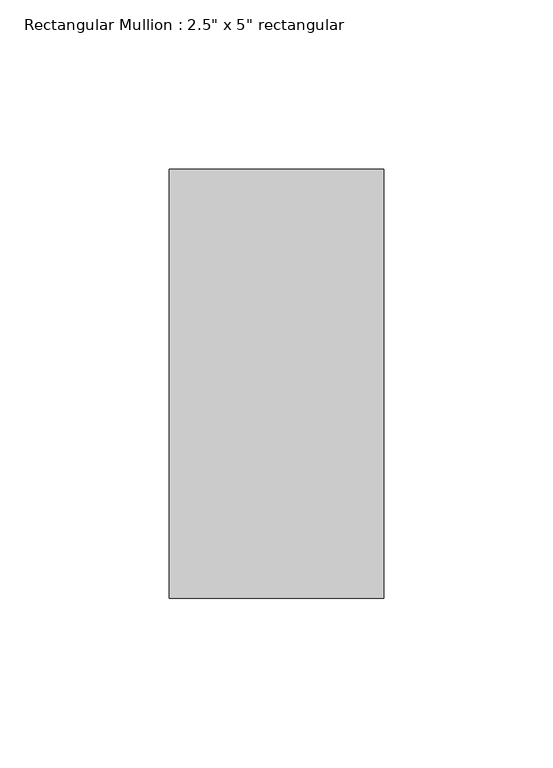
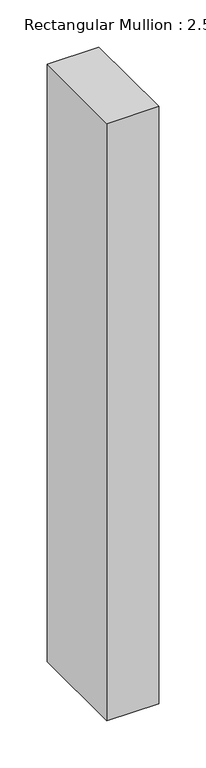
"""IFC4 building model written with IfcOpenShell, lengths in millimetres: member geometry."""

from ifc_helpers import new_model, si_unit, frame, origin, place, context, project, spatial, polyline, outline, extrude, source, transform, mapped, element, save


def member_972adede(model_context):
    return source(origin(), model_context, "Body", "SweptSolid", [
        extrude(outline(polyline([(0.0, 63.5), (0.0, -63.5), (-63.5, -63.5), (-63.5, 63.5), (0.0, 63.5)])), frame((0.0, 0.0, -774.7), z_axis=(0.0, 0.0, 1.0), x_axis=(1.0, 0.0, 0.0)), (0.0, 0.0, 1.0), 774.7),
    ])


if __name__ == "__main__":
    model = new_model("IFC4")
    model_context = context("Model", 3, world=origin())
    ifc_project = project(units=[si_unit("LENGTHUNIT", "METRE", prefix="MILLI")], contexts=[model_context])
    site = spatial("IfcSite", under=ifc_project)
    building = spatial("IfcBuilding", under=site)
    placement = place(None, origin())
    member_shape = member_972adede(model_context)
    element("IfcMember", 1, ObjectType="Rectangular Mullion : 2.5\" x 5\" rectangular", at=placement, inside=building, context=model_context, shape_type="MappedRepresentation", body=[
        mapped(member_shape, transform((0.0, 0.0, 0.0), x_axis=(1.0, 0.0, 0.0), y_axis=(0.0, 1.0, 0.0), z_axis=(0.0, 0.0, 1.0))),
    ])
    save(model, "model.ifc")

# Revit data of these elements
# Type "Rectangular Mullion : 2.5\" x 5\" rectangular"
#   built-in parameter 1007304 = 0.416667 (stored number, unit not read)
#   built-in parameter 1007301 = 0.104167 (stored number, unit not read)
#   built-in parameter 1007300 = 0.104167 (stored number, unit not read)
# Element 1 (IfcMember, "Rectangular Mullion : 2.5\" x 5\" rectangular")
#   Materials on its faces: "Aluminum"
# Materials
#   "Aluminum": class "Metal", colour RGB 247 247 247, transparency 0, Description = "Aluminum 6061", Cost = 0
